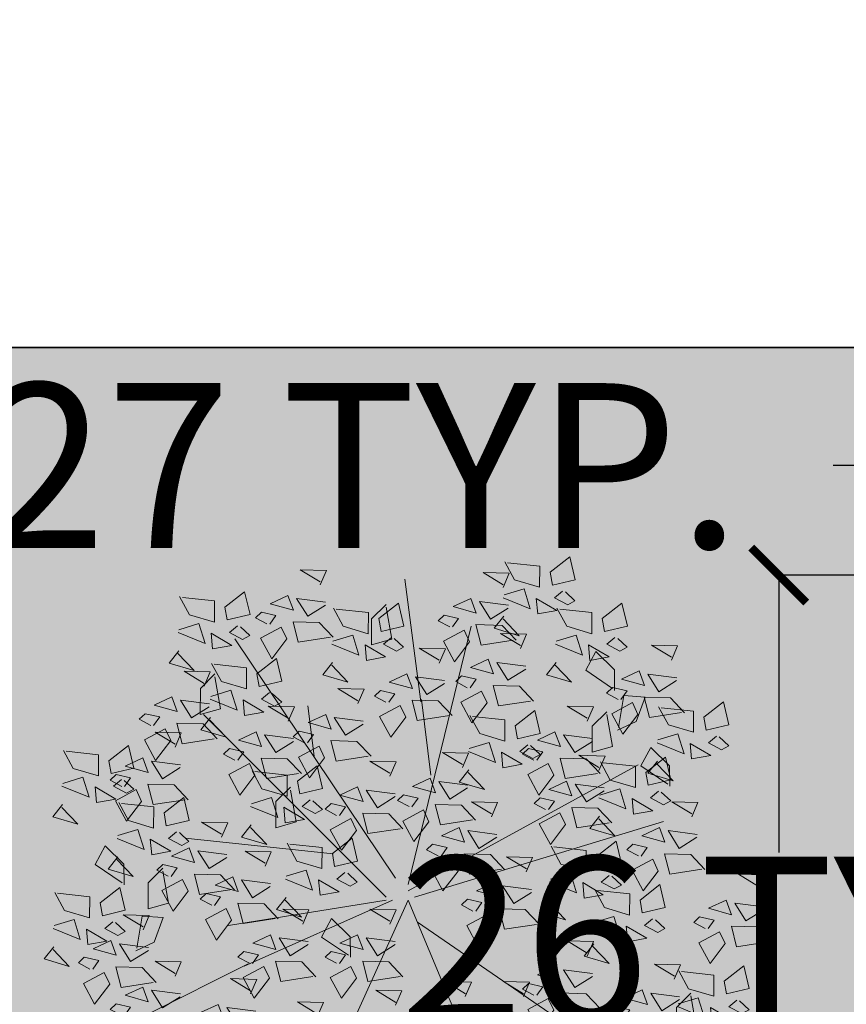
# Model space of a CAD drawing. Units: inches. Extents: x 1704 to 6393, y -157 to 1172.
# Tile 77 of 122: x 1987 to 2017, y 1009 to 1045. Entities that reach past the tile are written whole.
import ezdxf

# ---------------------------------------------------------------- set-up
doc = ezdxf.new("R2010")
doc.units = ezdxf.units.IN
doc.header["$MEASUREMENT"] = 0
for name, color, linetype, lineweight in [('A-ANNO-DIMS', 7, 'Continuous', 13), ('C-PROP', 7, 'Continuous', 35), ('L-shrub', 74, 'Continuous', 18)]:
    doc.layers.add(name, color=color, linetype=linetype, lineweight=lineweight)
doc.layers.add('L-HRDS-PATT', color=9, linetype='Continuous', lineweight=13, true_color=0xc5c1ba)
doc.styles.get("Standard").update_dxf_attribs({"font": 'arial.ttf'})
doc.dimstyles.get("Standard").update_dxf_attribs({"dimtxt": 6, "dimasz": 2, "dimexe": 0.18, "dimexo": 0.0625, "dimgap": 0.09, "dimtad": 0, "dimtih": 1, "dimtoh": 1, "dimdec": 1, "dimzin": 0, "dimdsep": 46, "dimlunit": 3, "dimtxsty": 'Standard', "dimblk": 'ARCHTICK', "dimcen": 0.09, "dimadec": 0, "dimazin": 0, "dimtfac": 1, "dimtdec": 1, "dimtofl": 0, "dimtmove": 0, "dimatfit": 3, "dimfxl": 1, "dimtolj": 1, "dimtzin": 0, "dimarcsym": 0})

# ---------------------------------------------------------------- blocks, each defined once
blk = doc.blocks.new('flower shrub 2')
at = {"layer": 'L-shrub'}
for p, q in [((-106.23, 211.82), (-92.99, 218)), ((-112.6, 194.32), (-106.23, 211.82)), ((-93.69, 216.06), (-97.6, 193.26)), ((-81.12, 192.39), (-66.64, 196.47)), ((-66.64, 196.47), (-66.71, 177.85)), ((71.95, 198.59), (86.43, 202.67)), ((75.99, 175.82), (71.95, 198.59)), ((86.43, 202.67), (86.36, 184.05)), ((-97.6, 193.26), (-112.6, 194.32)), ((-77.07, 169.62), (-81.12, 192.39)), ((86.36, 184.05), (75.99, 173.75)), ((-66.71, 177.85), (-77.08, 167.55)), ((26.45, 165.53), (40.92, 169.61)), ((40.92, 169.61), (40.85, 150.99)), ((-145.24, 163.47), (-130.76, 167.54)), ((-141.2, 140.7), (-145.24, 163.47)), ((-130.76, 167.54), (-130.83, 148.93)), ((-88.72, 152.29), (-88.87, 166.9)), ((-87.4, 165.46), (-68.26, 152.47)), ((30.49, 142.76), (26.45, 165.53)), ((60.21, 144.02), (60.06, 158.64)), ((61.53, 157.19), (80.67, 144.21)), ((-130.83, 148.93), (-141.21, 138.63)), ((-75.44, 139.25), (-88.72, 152.29)), ((-68.26, 152.47), (-75.44, 139.25)), ((40.85, 150.99), (30.48, 140.69)), ((73.5, 130.99), (60.21, 144.02)), ((80.67, 144.21), (73.5, 130.99)), ((-201.09, 93.22), (-186.61, 97.3)), ((-197.05, 70.45), (-201.09, 93.22)), ((-186.61, 97.3), (-186.68, 78.69)), ((-186.68, 78.69), (-197.06, 68.38)), ((45.73, 28.33), (45.58, 42.95)), ((47.06, 41.5), (66.19, 28.51)), ((185.43, 32.08), (198.67, 38.26)), ((197.96, 36.32), (194.06, 13.53)), ((59.02, 15.29), (45.73, 28.33)), ((66.19, 28.51), (59.02, 15.29)), ((179.06, 14.59), (185.43, 32.08)), ((194.06, 13.53), (179.06, 14.59)), ((175.38, 4.39), (189.86, 8.47)), ((189.86, 8.47), (189.78, -10.15)), ((179.42, -18.38), (175.38, 4.39)), ((189.78, -10.15), (179.41, -20.45)), ((207.07, -23.32), (206.92, -8.7)), ((208.4, -10.15), (227.53, -23.13)), ((220.36, -36.35), (207.07, -23.32)), ((227.53, -23.13), (220.36, -36.35)), ((84.36, -53.46), (98.84, -49.38)), ((88.41, -76.23), (84.36, -53.46)), ((98.84, -49.38), (98.77, -68)), ((98.77, -68), (88.4, -78.3)), ((-181.81, -93.56), (-181.96, -78.94)), ((-180.48, -80.39), (-161.34, -93.38)), ((-168.52, -106.6), (-181.81, -93.56)), ((-161.34, -93.38), (-168.52, -106.6)), ((-141.1, -107.17), (-126.62, -103.09)), ((-126.62, -103.09), (-126.7, -121.71)), ((-137.06, -129.94), (-141.1, -107.17)), ((-157.94, -124.93), (-144.7, -118.75)), ((-164.31, -142.42), (-157.94, -124.93)), ((-145.41, -120.69), (-149.31, -143.48)), ((-126.7, -121.71), (-137.07, -132.01)), ((138.15, -134.03), (152.62, -129.95)), ((152.62, -129.95), (152.55, -148.57)), ((142.19, -156.8), (138.15, -134.03)), ((-149.31, -143.48), (-164.31, -142.42)), ((-142.51, -161.74), (-142.65, -147.12)), ((-141.18, -148.57), (-122.04, -161.55)), ((152.55, -148.57), (142.18, -158.87)), ((-129.22, -174.77), (-142.51, -161.74)), ((-122.04, -161.55), (-129.22, -174.77)), ((16.1, -183.61), (30.58, -179.53)), ((30.58, -179.53), (30.51, -198.15)), ((20.14, -206.38), (16.1, -183.61)), ((30.51, -198.15), (20.14, -208.45))]:
    blk.add_line(p, q, dxfattribs=at)
for points in [[(52.15, 237.83), (59.05, 246.56), (41.2, 251.84), (52.74, 239.81)], [(-67.82, 227.5), (-60.92, 236.23), (-78.77, 241.51), (-67.23, 229.48)], [(-39.32, 221.12), (-28.59, 235.29), (-20.71, 220.61), (-35.41, 212.74), (-39.32, 221.12)], [(29.03, 225.28), (27.99, 236.36), (14.33, 233.94), (29.03, 225.28)], [(52.02, 222.79), (37.77, 218.39), (33.35, 232.62), (52.6, 224.77)], [(-90.95, 214.95), (-91.98, 226.03), (-105.64, 223.61), (-90.95, 214.95)], [(10.23, 220.07), (15.95, 224.84), (6.62, 229.76), (1.48, 226.97), (8.24, 220.66)], [(126.62, 210.97), (133.52, 219.7), (115.67, 224.99), (127.2, 212.95)], [(-109.75, 209.74), (-104.02, 214.51), (-113.35, 219.43), (-118.49, 216.64), (-111.73, 210.33)], [(-67.96, 212.46), (-82.2, 208.06), (-86.62, 222.29), (-67.37, 214.44)], [(-70.39, 219.89), (-47.54, 223.41), (-43.79, 208.84), (-62.4, 209.34), (-72.46, 219.95)], [(-27.19, 210.46), (-31.5, 204.37), (-21.21, 202.03), (-16.97, 206.05), (-25.13, 210.4)], [(19.2, 206.65), (5.18, 195.71), (1.34, 211.93), (17.57, 215.74), (19.2, 206.65)], [(49.53, 199.82), (26.54, 202.32), (26.68, 217.36), (44.53, 212.08), (51.52, 199.24)], [(-100.78, 196.32), (-114.8, 185.38), (-118.63, 201.6), (-102.4, 205.41), (-100.78, 196.32)], [(-70.44, 189.49), (-93.43, 191.99), (-93.29, 207.03), (-75.44, 201.75), (-68.45, 188.91)], [(-66.87, 197.06), (-54.24, 204.99), (-46.3, 192.37), (-66.93, 195)], [(16.53, 190.13), (27.26, 204.31), (35.14, 189.63), (20.44, 181.76), (16.53, 190.13)], [(103.49, 198.43), (102.46, 209.5), (88.8, 207.08), (103.49, 198.43)], [(126.48, 195.93), (112.24, 191.53), (107.82, 205.76), (127.07, 197.91)], [(-47.57, 123.92), (-79, 197.93)], [(-44.01, 200.58), (-40.16, 190.14), (-27.58, 196), (-44.01, 200.58)], [(-37.25, 183.93), (-26.52, 198.11), (-18.64, 183.43), (-33.34, 175.56), (-37.25, 183.93)], [(84.69, 193.22), (90.42, 197.99), (81.09, 202.9), (75.95, 200.11), (82.71, 193.8)], [(-136.54, 179.8), (-125.81, 193.98), (-117.93, 179.3), (-132.63, 171.43), (-136.54, 179.8)], [(-14.54, 188.9), (8.31, 192.42), (12.06, 177.85), (-6.55, 178.35), (-16.61, 188.96)], [(124, 172.97), (101.01, 175.46), (101.15, 190.5), (119, 185.22), (125.98, 172.38)], [(-68.32, 182.7), (-45.47, 186.22), (-41.72, 171.65), (-60.33, 172.15), (-70.39, 182.76)], [(-63.13, 182.49), (-67.54, 172.28), (-48.93, 171.78), (-63.18, 180.43)], [(64.56, 171.72), (71.46, 180.45), (53.61, 185.73), (65.15, 173.7)], [(93.66, 179.79), (79.64, 168.86), (75.81, 185.07), (92.04, 188.89), (93.66, 179.79)], [(-167.61, 178.57), (-144.76, 182.09), (-141.01, 167.52), (-159.62, 168.02), (-169.68, 178.63)], [(28.66, 179.47), (24.35, 173.38), (34.64, 171.04), (38.88, 175.06), (30.72, 179.41)], [(66.94, 139.62), (91.63, 182.23)], [(141.1, 161.39), (148, 170.12), (130.14, 175.4), (141.68, 163.37)], [(-124.41, 169.14), (-128.72, 163.05), (-118.43, 160.71), (-114.19, 164.73), (-122.34, 169.08)], [(-78.16, 157.26), (-71.26, 165.99), (-89.12, 171.27), (-77.58, 159.24)], [(-25.12, 173.27), (-29.43, 167.19), (-19.14, 164.84), (-14.9, 168.86), (-23.06, 173.21)], [(-11.02, 166.07), (1.61, 174), (9.54, 161.38), (-11.08, 164.01)], [(11.84, 169.59), (15.69, 159.15), (28.27, 165.01), (11.84, 169.59)], [(41.44, 159.17), (40.4, 170.25), (26.74, 167.83), (41.44, 159.17)], [(-164.09, 155.74), (-151.46, 163.67), (-143.52, 151.05), (-164.15, 153.68)], [(-105.51, 148.81), (-94.78, 162.99), (-86.9, 148.31), (-101.6, 140.44), (-105.51, 148.81)], [(-64.8, 159.87), (-52.17, 167.8), (-44.24, 155.19), (-64.86, 157.81)], [(-41.95, 163.39), (-38.09, 152.95), (-25.52, 158.81), (-41.95, 163.39)], [(22.64, 153.96), (28.36, 158.73), (19.03, 163.65), (13.89, 160.86), (20.65, 154.55)], [(64.43, 156.68), (50.18, 152.28), (45.76, 166.51), (65.01, 158.66)], [(207.29, 148.99), (214.19, 157.72), (196.34, 163.01), (207.88, 150.97)], [(-165.04, 146.93), (-158.14, 155.66), (-175.99, 160.94), (-164.45, 148.91)], [(-141.23, 159.26), (-137.38, 148.82), (-124.8, 154.68), (-141.23, 159.26)], [(-101.29, 144.71), (-102.33, 155.79), (-115.98, 153.37), (-101.29, 144.71)], [(117.97, 148.84), (116.93, 159.92), (103.28, 157.5), (117.97, 148.84)], [(140.96, 146.35), (126.72, 141.95), (122.3, 156.18), (141.55, 148.33)], [(-136.58, 147.58), (-113.73, 151.1), (-109.98, 136.53), (-128.59, 137.03), (-138.65, 147.64)], [(-120.09, 139.5), (-114.36, 144.27), (-123.69, 149.19), (-128.83, 146.4), (-122.07, 140.09)], [(-78.3, 142.22), (-92.54, 137.81), (-96.96, 152.05), (-77.71, 144.2)], [(-7.28, 151.5), (-11.69, 141.29), (6.92, 140.79), (-7.33, 149.44)], [(31.61, 140.54), (17.59, 129.6), (13.76, 145.82), (29.99, 149.63), (31.61, 140.54)], [(61.95, 133.71), (38.95, 136.21), (39.09, 151.25), (56.94, 145.97), (63.93, 133.13)], [(99.17, 143.63), (104.9, 148.4), (95.57, 153.32), (90.43, 150.53), (97.19, 144.22)], [(184.16, 136.45), (183.13, 147.53), (169.47, 145.1), (184.16, 136.45)], [(-188.17, 134.38), (-189.2, 145.46), (-202.86, 143.04), (-188.17, 134.38)], [(-165.18, 131.89), (-179.42, 127.48), (-183.84, 141.72), (-164.59, 133.87)], [(-160.34, 141.17), (-164.76, 130.96), (-146.15, 130.46), (-160.4, 139.11)], [(-61.06, 145.31), (-65.47, 135.09), (-46.86, 134.59), (-61.11, 143.24)], [(138.48, 123.38), (115.49, 125.88), (115.63, 140.92), (133.48, 135.64), (140.46, 122.8)], [(165.36, 131.24), (171.09, 136.01), (161.76, 140.92), (156.62, 138.13), (163.38, 131.82)], [(207.15, 133.95), (192.91, 129.55), (188.49, 143.78), (207.74, 135.93)], [(-206.97, 129.17), (-201.24, 133.94), (-210.57, 138.86), (-215.71, 136.07), (-208.95, 129.76)], [(-111.12, 126.07), (-125.14, 115.14), (-128.97, 131.36), (-112.74, 135.17), (-111.12, 126.07)], [(-80.78, 119.25), (-103.77, 121.75), (-103.63, 136.79), (-85.78, 131.5), (-78.8, 118.66)], [(-93.39, 138.15), (-97.69, 132.06), (-87.4, 129.72), (-83.16, 133.74), (-91.32, 138.09)], [(108.14, 130.21), (94.12, 119.27), (90.29, 135.49), (106.52, 139.3), (108.14, 130.21)], [(93.06, 124.02), (103.79, 138.2), (111.67, 123.52), (96.98, 115.65), (93.06, 124.02)], [(-167.66, 108.92), (-190.65, 111.42), (-190.51, 126.46), (-172.66, 121.17), (-165.67, 108.33)], [(-133.06, 124.75), (-120.43, 132.68), (-112.5, 120.06), (-133.12, 122.69)], [(-110.21, 128.27), (-106.35, 117.83), (-93.78, 123.69), (-110.21, 128.27)], [(37.21, 115.75), (47.94, 129.93), (55.82, 115.25), (41.13, 107.38), (37.21, 115.75)], [(61.99, 122.79), (84.85, 126.31), (88.59, 111.74), (69.98, 112.24), (59.92, 122.85)], [(174.33, 117.81), (160.31, 106.88), (156.48, 123.09), (172.71, 126.91), (174.33, 117.81)], [(204.67, 110.99), (181.68, 113.48), (181.82, 128.52), (199.67, 123.24), (206.65, 110.4)], [(-198, 115.75), (-212.02, 104.81), (-215.85, 121.03), (-199.62, 124.84), (-198, 115.75)], [(-53.8, 109.56), (-43.07, 123.73), (-35.19, 109.05), (-49.89, 101.18), (-53.8, 109.56)], [(-12.43, 109.56), (-1.7, 123.73), (6.18, 109.05), (-8.52, 101.18), (-12.43, 109.56)], [(4.49, 2.24), (58.38, 121.09)], [(140.64, 107.49), (151.37, 121.67), (159.25, 106.99), (144.55, 99.12), (140.64, 107.49)], [(-2.25, 17.94), (-145.94, 116.61)], [(6.14, 114.53), (29, 118.04), (32.74, 103.47), (14.13, 103.98), (4.07, 114.58)], [(105.19, 113.36), (100.89, 107.27), (111.17, 104.93), (115.42, 108.95), (107.26, 113.3)], [(-161.36, 97.16), (-150.63, 111.34), (-142.75, 96.66), (-157.45, 88.79), (-161.36, 97.16)], [(-129.32, 110.18), (-133.73, 99.97), (-115.12, 99.47), (-129.37, 108.12)], [(-84.87, 108.33), (-62.02, 111.85), (-58.27, 97.28), (-76.88, 97.78), (-86.94, 108.38)], [(-43.5, 108.33), (-20.65, 111.85), (-16.9, 97.28), (-35.51, 97.78), (-45.57, 108.38)], [(4.49, 2.24), (-40.41, 109.88)], [(65.51, 99.96), (78.14, 107.89), (86.08, 95.27), (65.46, 97.9)], [(109.57, 106.26), (132.42, 109.78), (136.17, 95.21), (117.56, 95.71), (107.5, 106.32)], [(194.42, 95.09), (205.15, 109.27), (213.03, 94.59), (198.33, 86.72), (194.42, 95.09)], [(-187.79, 91.15), (-180.89, 99.88), (-198.75, 105.16), (-187.21, 93.13)], [(-192.43, 95.93), (-169.58, 99.45), (-165.83, 84.88), (-184.44, 85.38), (-194.5, 95.99)], [(-41.67, 98.9), (-45.98, 92.81), (-35.69, 90.47), (-31.45, 94.49), (-39.6, 98.84)], [(-0.3, 98.9), (-4.61, 92.81), (5.68, 90.47), (9.92, 94.49), (1.76, 98.84)], [(9.66, 91.7), (22.29, 99.62), (30.23, 87.01), (9.61, 89.63)], [(49.34, 105.09), (45.04, 99.01), (55.32, 96.67), (59.57, 100.68), (51.41, 105.04)], [(88.37, 103.48), (92.23, 93.04), (104.8, 98.9), (88.37, 103.48)], [(-99.31, 80.63), (-88.58, 94.81), (-80.7, 80.13), (-95.39, 72.26), (-99.31, 80.63)], [(-81.35, 85.5), (-68.72, 93.43), (-60.78, 80.81), (-81.41, 83.43)], [(-39.98, 85.5), (-27.35, 93.43), (-19.41, 80.81), (-40.04, 83.43)], [(32.52, 95.21), (36.38, 84.78), (48.95, 90.64), (32.52, 95.21)], [(113.09, 83.43), (125.72, 91.36), (133.65, 78.75), (113.03, 81.37)], [(152.77, 96.83), (148.46, 90.75), (158.75, 88.4), (162.99, 92.42), (154.83, 96.77)], [(163.35, 93.87), (186.2, 97.38), (189.95, 82.82), (171.34, 83.32), (161.28, 93.92)], [(-210.92, 78.6), (-211.96, 89.68), (-225.62, 87.26), (-210.92, 78.6)], [(-187.93, 76.11), (-202.17, 71.7), (-206.59, 85.94), (-187.34, 78.09)], [(-149.23, 86.5), (-153.54, 80.42), (-143.25, 78.07), (-139.01, 82.09), (-147.17, 86.44)], [(-58.49, 89.02), (-54.64, 78.58), (-42.06, 84.44), (-58.49, 89.02)], [(-17.12, 89.02), (-13.27, 78.58), (-0.69, 84.44), (-17.12, 89.02)], [(69.26, 85.39), (64.84, 75.18), (83.45, 74.68), (69.2, 83.33)], [(135.94, 86.95), (139.8, 76.51), (152.38, 82.37), (135.94, 86.95)], [(206.55, 84.43), (202.24, 78.35), (212.53, 76.01), (216.77, 80.02), (208.61, 84.38)], [(-229.72, 73.39), (-223.99, 78.16), (-233.32, 83.08), (-238.46, 80.29), (-231.7, 73.98)], [(-188.91, 73.1), (-176.28, 81.03), (-168.35, 68.42), (-188.97, 71.04)], [(-130.38, 79.41), (-107.52, 82.92), (-103.78, 68.35), (-122.39, 68.86), (-132.45, 79.46)], [(118.58, 47.68), (190.43, 83.56)], [(166.87, 71.04), (179.5, 78.96), (187.44, 66.35), (166.81, 68.97)], [(-190.41, 53.14), (-213.4, 55.64), (-213.26, 70.68), (-195.41, 65.39), (-188.43, 52.55)], [(-166.05, 76.62), (-162.2, 66.18), (-149.62, 72.04), (-166.05, 76.62)], [(-77.6, 70.93), (-82.02, 60.72), (-63.41, 60.22), (-77.66, 68.87)], [(-36.23, 70.93), (-40.65, 60.72), (-22.04, 60.22), (-36.29, 68.87)], [(13.41, 77.13), (8.99, 66.92), (27.6, 66.41), (13.35, 75.06)], [(41.35, 57.91), (52.08, 72.09), (59.96, 57.41), (45.26, 49.54), (41.35, 57.91)], [(103.41, 57.91), (114.13, 72.09), (122.01, 57.41), (107.32, 49.54), (103.41, 57.91)], [(189.73, 74.55), (193.58, 64.12), (206.16, 69.98), (189.73, 74.55)], [(217.17, 62.04), (227.9, 76.22), (235.78, 61.54), (221.08, 53.67), (217.17, 62.04)], [(-220.75, 59.96), (-234.77, 49.03), (-238.6, 65.25), (-222.37, 69.06), (-220.75, 59.96)], [(-126.86, 56.58), (-114.23, 64.5), (-106.29, 51.89), (-126.91, 54.51)], [(-87.18, 69.97), (-91.48, 63.89), (-81.2, 61.54), (-76.95, 65.56), (-85.11, 69.92)], [(116.83, 68.87), (112.42, 58.65), (131.03, 58.15), (116.78, 66.8)], [(186.1, 60.81), (208.96, 64.33), (212.7, 49.76), (194.09, 50.26), (184.03, 60.87)], [(-185.17, 58.54), (-189.58, 48.32), (-170.97, 47.82), (-185.22, 56.47)], [(-104, 60.09), (-100.14, 49.66), (-87.57, 55.52), (-104, 60.09)], [(10.28, 56.68), (33.14, 60.2), (36.88, 45.63), (18.27, 46.13), (8.21, 56.74)], [(72.33, 56.68), (95.19, 60.2), (98.94, 45.63), (80.33, 46.13), (70.27, 56.74)], [(170.61, 56.47), (166.2, 46.26), (184.81, 45.75), (170.56, 54.41)], [(15.72, 2.24), (121.24, 49.33)], [(229.3, 51.38), (225, 45.3), (235.28, 42.95), (239.53, 46.97), (231.37, 51.32)], [(256.93, 35.37), (263.83, 44.1), (245.98, 49.38), (257.52, 37.35)], [(-221.35, 33.12), (-210.62, 47.29), (-202.74, 32.61), (-217.44, 24.74), (-221.35, 33.12)], [(-127.81, 33.3), (-120.91, 42.03), (-138.76, 47.31), (-127.22, 35.28)], [(53.48, 47.25), (49.18, 41.16), (59.46, 38.82), (63.71, 42.84), (55.55, 47.19)], [(115.53, 47.25), (111.23, 41.16), (121.51, 38.82), (125.76, 42.84), (117.6, 47.19)], [(189.62, 37.98), (202.25, 45.91), (210.19, 33.29), (189.57, 35.92)], [(-252.42, 31.89), (-229.56, 35.41), (-225.82, 20.84), (-244.43, 21.34), (-254.49, 31.94)], [(-123.11, 42.01), (-127.53, 31.79), (-108.92, 31.29), (-123.17, 39.94)], [(13.8, 33.85), (26.43, 41.78), (34.37, 29.16), (13.74, 31.79)], [(36.66, 37.37), (40.51, 26.93), (53.09, 32.79), (36.66, 37.37)], [(75.86, 33.85), (88.48, 41.78), (96.42, 29.16), (75.8, 31.79)], [(98.71, 37.37), (102.57, 26.93), (115.14, 32.79), (98.71, 37.37)], [(212.48, 41.5), (216.34, 31.06), (228.91, 36.92), (212.48, 41.5)], [(-150.93, 20.75), (-151.97, 31.83), (-165.63, 29.41), (-150.93, 20.75)], [(-127.94, 18.26), (-142.19, 13.86), (-146.61, 28.09), (-127.36, 20.24)], [(-55.87, 20.72), (-45.14, 34.9), (-37.26, 20.22), (-51.96, 12.35), (-55.87, 20.72)], [(130.3, 16.59), (141.02, 30.77), (148.91, 16.09), (134.21, 8.22), (130.3, 16.59)], [(233.81, 22.82), (232.77, 33.9), (219.11, 31.48), (233.81, 22.82)], [(256.8, 20.33), (242.55, 15.92), (238.13, 30.16), (257.38, 22.31)], [(-209.22, 22.46), (-213.52, 16.37), (-203.24, 14.03), (-198.99, 18.05), (-207.15, 22.4)], [(-169.73, 15.55), (-164.01, 20.31), (-173.34, 25.23), (-178.48, 22.44), (-171.72, 16.13)], [(-86.94, 19.49), (-64.08, 23.01), (-60.34, 8.44), (-78.95, 8.94), (-89.01, 19.55)], [(193.37, 23.42), (188.95, 13.2), (207.56, 12.7), (193.31, 21.35)], [(215.01, 17.61), (220.73, 22.38), (211.4, 27.3), (206.26, 24.51), (213.02, 18.2)], [(-248.9, 9.06), (-236.27, 16.99), (-228.33, 4.37), (-248.95, 7)], [(-96.78, 2.31), (-89.88, 11.04), (-107.73, 16.33), (-96.19, 4.29)], [(17.55, 19.28), (13.13, 9.07), (31.74, 8.57), (17.49, 17.22)], [(20.21, 2.24), (132.47, 20.18)], [(79.6, 19.28), (75.19, 9.07), (93.8, 8.57), (79.54, 17.22)], [(91.45, 0.25), (98.35, 8.98), (80.5, 14.26), (92.04, 2.23)], [(99.22, 15.36), (122.08, 18.88), (125.83, 4.31), (107.22, 4.81), (97.16, 15.42)], [(254.32, -2.64), (231.32, -0.14), (231.46, 14.9), (249.31, 9.61), (256.3, -3.23)], [(-226.04, 12.58), (-222.18, 2.14), (-209.61, 8), (-226.04, 12.58)], [(-160.76, 2.12), (-174.78, -8.81), (-178.61, 7.4), (-162.38, 11.22), (-160.76, 2.12)], [(-130.42, -4.7), (-153.42, -2.21), (-153.28, 12.83), (-135.43, 7.55), (-128.44, -5.29)], [(-43.74, 10.06), (-48.04, 3.98), (-37.76, 1.63), (-33.51, 5.65), (-41.67, 10)], [(161.32, -4.07), (172.05, 10.11), (179.93, -4.57), (165.24, -12.44), (161.32, -4.07)], [(223.98, 4.18), (209.96, -6.75), (206.13, 9.47), (222.35, 13.28), (223.98, 4.18)], [(0, 0), (-177.37, -53.82)], [(-119.91, -10.23), (-120.94, 0.84), (-134.6, -1.58), (-119.91, -10.23)], [(-83.42, -3.34), (-70.79, 4.59), (-62.85, -8.02), (-83.47, -5.4)], [(-60.56, 0.18), (-56.71, -10.26), (-44.13, -4.4), (-60.56, 0.18)], [(20.21, 0), (150.43, -130.06)], [(102.75, -7.47), (115.38, 0.46), (123.31, -12.16), (102.69, -9.53)], [(142.42, 5.93), (138.12, -0.16), (148.4, -2.5), (152.65, 1.52), (144.49, 5.87)], [(-245.15, -5.51), (-249.57, -15.72), (-230.96, -16.22), (-245.21, -7.57)], [(-173.77, -18.53), (-163.04, -4.35), (-155.16, -19.03), (-169.86, -26.9), (-173.77, -18.53)], [(4.49, -4.48), (-159.41, -94.18)], [(-138.71, -15.44), (-132.98, -10.67), (-142.31, -5.76), (-147.45, -8.55), (-140.69, -14.86)], [(-96.92, -12.73), (-111.16, -17.13), (-115.58, -2.9), (-96.33, -10.75)], [(-31.05, -18.53), (-20.32, -4.35), (-12.44, -19.03), (-27.13, -26.9), (-31.05, -18.53)], [(68.33, -12.3), (67.29, -1.22), (53.63, -3.64), (68.33, -12.3)], [(91.32, -14.79), (77.07, -19.2), (72.66, -4.96), (91.9, -12.81)], [(125.6, -3.95), (129.46, -14.39), (142.03, -8.53), (125.6, -3.95)], [(130.25, -5.3), (153.11, -1.78), (156.85, -16.35), (138.24, -15.85), (128.18, -5.24)], [(4.49, -8.97), (-40.41, -192.85)], [(13.47, -13.45), (127.98, -183.88)], [(49.53, -17.51), (55.25, -12.74), (45.92, -7.82), (40.78, -10.61), (47.54, -16.92)], [(-204.84, -19.76), (-181.99, -16.24), (-178.24, -30.81), (-196.85, -30.31), (-206.91, -19.7)], [(-129.74, -28.87), (-143.76, -39.8), (-147.59, -23.59), (-131.36, -19.77), (-129.74, -28.87)], [(-99.4, -35.69), (-122.39, -33.2), (-122.25, -18.16), (-104.4, -23.44), (-97.41, -36.28)], [(-79.67, -17.9), (-84.09, -28.12), (-65.48, -28.62), (-79.73, -19.97)], [(-62.12, -19.76), (-39.26, -16.24), (-35.52, -30.81), (-54.13, -30.31), (-64.19, -19.7)], [(88.84, -37.76), (65.84, -35.27), (65.98, -20.22), (83.83, -25.51), (90.82, -38.35)], [(133.77, -28.13), (146.4, -20.2), (154.34, -32.82), (133.72, -30.19)], [(173.45, -14.73), (169.15, -20.81), (179.43, -23.16), (183.68, -19.14), (175.52, -14.79)], [(211.43, -28.68), (218.32, -19.95), (200.47, -14.66), (212.01, -26.7)], [(58.5, -30.94), (44.48, -41.87), (40.65, -25.65), (56.88, -21.84), (58.5, -30.94)], [(106.49, -22.04), (102.08, -32.25), (120.69, -32.75), (106.44, -24.1)], [(156.63, -24.61), (160.49, -35.05), (173.06, -29.19), (156.63, -24.61)], [(-201.32, -42.59), (-188.69, -34.66), (-180.76, -47.28), (-201.38, -44.65)], [(-161.65, -29.19), (-165.95, -35.28), (-155.67, -37.62), (-151.42, -33.6), (-159.58, -29.25)], [(-58.6, -42.59), (-45.97, -34.66), (-38.03, -47.28), (-58.65, -44.65)], [(-18.92, -29.19), (-23.22, -35.28), (-12.94, -37.62), (-8.69, -33.6), (-16.85, -29.25)], [(41.35, -47.45), (52.08, -33.28), (59.96, -47.96), (45.26, -55.83), (41.35, -47.45)], [(57.96, -30.81), (163.48, -42.02)], [(188.3, -41.22), (187.26, -30.14), (173.6, -32.57), (188.3, -41.22)], [(211.29, -43.72), (197.04, -48.12), (192.63, -33.89), (211.88, -41.74)], [(-178.47, -39.07), (-174.61, -49.51), (-162.04, -43.65), (-178.47, -39.07)], [(-107.58, -51.59), (-96.85, -37.41), (-88.97, -52.09), (-103.67, -59.96), (-107.58, -51.59)], [(-35.74, -39.07), (-31.88, -49.51), (-19.31, -43.65), (-35.74, -39.07)], [(-10.36, -53.65), (0.37, -39.48), (8.25, -54.15), (-6.45, -62.02), (-10.36, -53.65)], [(116.28, -51.4), (123.17, -42.67), (105.32, -37.39), (116.86, -49.42)], [(169.5, -46.43), (175.23, -41.66), (165.89, -36.75), (160.76, -39.54), (167.52, -45.85)], [(-131.94, -57.6), (-125.04, -48.87), (-142.9, -43.59), (-131.36, -55.62)], [(10.28, -48.68), (33.14, -45.17), (36.88, -59.73), (18.27, -59.23), (8.21, -48.63)], [(137.52, -42.69), (133.1, -52.91), (151.71, -53.41), (137.46, -44.76)], [(-138.65, -52.81), (-115.8, -49.3), (-112.05, -63.87), (-130.66, -63.36), (-140.72, -52.76)], [(-41.43, -54.88), (-18.58, -51.36), (-14.83, -65.93), (-33.44, -65.43), (-43.5, -54.82)], [(93.15, -63.95), (92.11, -52.87), (78.45, -55.29), (93.15, -63.95)], [(178.47, -59.86), (164.45, -70.79), (160.62, -54.58), (176.85, -50.76), (178.47, -59.86)], [(208.81, -66.68), (185.82, -64.19), (185.95, -49.15), (203.81, -54.43), (210.79, -67.27)], [(194.42, -68.11), (205.15, -53.94), (213.03, -68.62), (198.33, -76.49), (194.42, -68.11)], [(250.73, -65.86), (257.63, -57.13), (239.78, -51.85), (251.31, -63.88)], [(-197.58, -57.16), (-201.99, -67.37), (-183.38, -67.87), (-197.63, -59.22)], [(-155.07, -70.15), (-156.11, -59.07), (-169.77, -61.49), (-155.07, -70.15)], [(-132.08, -72.64), (-146.33, -77.04), (-150.74, -62.81), (-131.49, -70.66)], [(-95.45, -62.25), (-99.76, -68.33), (-89.47, -70.68), (-85.23, -66.66), (-93.39, -62.3)], [(-54.85, -57.16), (-59.27, -67.37), (-40.66, -67.87), (-54.91, -59.22)], [(53.48, -58.12), (49.18, -64.2), (59.46, -66.54), (63.71, -62.52), (55.55, -58.17)], [(74.35, -69.16), (80.08, -64.39), (70.74, -59.47), (65.6, -62.26), (72.37, -68.57)], [(116.14, -66.44), (101.89, -70.85), (97.48, -56.61), (116.73, -64.46)], [(-173.87, -75.36), (-168.14, -70.59), (-177.47, -65.67), (-182.61, -68.46), (-175.85, -74.77)], [(-135.13, -75.64), (-122.5, -67.72), (-114.56, -80.33), (-135.19, -77.71)], [(-37.91, -77.71), (-25.28, -69.78), (-17.35, -82.4), (-37.97, -79.77)], [(1.77, -64.31), (-2.54, -70.4), (7.75, -72.74), (11.99, -68.72), (3.83, -64.37)], [(13.8, -71.51), (26.43, -63.59), (34.37, -76.2), (13.74, -73.58)], [(36.66, -67.99), (40.51, -78.43), (53.09, -72.57), (36.66, -67.99)], [(163.35, -69.34), (186.2, -65.83), (189.95, -80.39), (171.34, -79.89), (161.28, -69.29)], [(227.6, -78.41), (226.56, -67.33), (212.91, -69.75), (227.6, -78.41)], [(-112.27, -72.13), (-108.42, -82.56), (-95.84, -76.7), (-112.27, -72.13)], [(-99.31, -86.71), (-88.58, -72.53), (-80.7, -87.21), (-95.39, -95.08), (-99.31, -86.71)], [(-38.86, -90.66), (-31.96, -81.92), (-49.81, -76.64), (-38.27, -88.67)], [(-15.06, -74.19), (-11.2, -84.63), (1.38, -78.77), (-15.06, -74.19)], [(83.32, -82.58), (69.3, -93.52), (65.47, -77.3), (81.7, -73.49), (83.32, -82.58)], [(113.66, -89.41), (90.67, -86.91), (90.8, -71.87), (108.65, -77.16), (115.64, -90)], [(113.75, -86.71), (124.48, -72.53), (132.36, -87.21), (117.66, -95.08), (113.75, -86.71)], [(208.8, -83.62), (214.53, -78.85), (205.2, -73.93), (200.06, -76.72), (206.82, -83.03)], [(250.59, -80.9), (236.35, -85.31), (231.93, -71.07), (251.18, -78.92)], [(-173.31, -96.85), (-166.41, -88.12), (-184.27, -82.84), (-172.73, -94.87)], [(-164.9, -88.78), (-178.92, -99.72), (-182.75, -83.5), (-166.52, -79.68), (-164.9, -88.78)], [(-134.56, -95.61), (-157.55, -93.11), (-157.42, -78.07), (-139.56, -83.35), (-132.58, -96.19)], [(206.55, -78.77), (202.24, -84.86), (212.53, -87.2), (216.77, -83.18), (208.61, -78.83)], [(-131.39, -90.21), (-135.8, -100.43), (-117.19, -100.93), (-131.44, -92.28)], [(-130.38, -87.94), (-107.52, -84.42), (-103.78, -98.99), (-122.39, -98.48), (-132.45, -87.88)], [(-4.91, -140.69), (-11.65, -86.87)], [(17.55, -86.08), (13.13, -96.29), (31.74, -96.8), (17.49, -88.14)], [(64.1, -99.1), (74.83, -84.93), (82.71, -99.61), (68.02, -107.48), (64.1, -99.1)], [(82.68, -87.94), (105.53, -84.42), (109.28, -98.99), (90.67, -98.48), (80.61, -87.88)], [(166.87, -92.17), (179.5, -84.24), (187.44, -96.86), (166.81, -94.24)], [(189.73, -88.65), (193.58, -99.09), (206.16, -93.23), (189.73, -88.65)], [(217.77, -97.05), (203.75, -107.98), (199.92, -91.76), (216.15, -87.95), (217.77, -97.05)], [(248.11, -103.87), (225.12, -101.38), (225.26, -86.33), (243.11, -91.62), (250.09, -104.46)], [(-87.18, -97.37), (-91.48, -103.45), (-81.2, -105.8), (-76.95, -101.78), (-85.11, -97.42)], [(-61.99, -103.2), (-63.02, -92.12), (-76.68, -94.54), (-61.99, -103.2)], [(-39, -105.7), (-53.24, -110.1), (-57.66, -95.86), (-38.41, -103.72)], [(-34.17, -92.28), (-38.58, -102.49), (-19.97, -102.99), (-34.22, -94.34)], [(33.03, -100.33), (55.89, -96.81), (59.63, -111.38), (41.02, -110.88), (30.96, -100.28)], [(125.88, -97.37), (121.57, -103.45), (131.86, -105.8), (136.1, -101.78), (127.94, -97.42)], [(173.73, -111.5), (184.46, -97.32), (192.34, -112), (177.65, -119.87), (173.73, -111.5)], [(-215.24, -114.61), (-209.51, -109.84), (-218.84, -104.92), (-223.98, -107.71), (-217.22, -114.02)], [(-196.44, -109.4), (-197.48, -98.32), (-211.14, -100.74), (-196.44, -109.4)], [(-173.45, -111.89), (-187.7, -116.3), (-192.11, -102.06), (-172.86, -109.91)], [(-126.86, -110.76), (-114.23, -102.84), (-106.29, -115.45), (-126.91, -112.83)], [(-80.79, -108.41), (-75.06, -103.64), (-84.39, -98.73), (-89.53, -101.51), (-82.77, -107.82)], [(71.43, -100.32), (75.92, -136.2)], [(86.2, -110.76), (98.83, -102.84), (106.76, -115.45), (86.14, -112.83)], [(-104, -107.25), (-100.14, -117.69), (-87.57, -111.82), (-104, -107.25)], [(-41.48, -128.66), (-64.47, -126.17), (-64.33, -111.13), (-46.48, -116.41), (-39.5, -129.25)], [(76.23, -109.76), (71.93, -115.85), (82.21, -118.19), (86.46, -114.17), (78.3, -109.82)], [(109.05, -107.25), (112.91, -117.69), (125.48, -111.82), (109.05, -107.25)], [(142.66, -112.73), (165.52, -109.21), (169.26, -123.78), (150.65, -123.28), (140.59, -112.67)], [(170.61, -106.74), (166.2, -116.95), (184.81, -117.46), (170.56, -108.8)], [(-206.27, -128.04), (-220.29, -138.97), (-224.12, -122.75), (-207.89, -118.94), (-206.27, -128.04)], [(-175.93, -134.86), (-198.92, -132.36), (-198.79, -117.32), (-180.93, -122.61), (-173.95, -135.45)], [(-159.29, -130.09), (-148.56, -115.91), (-140.68, -130.59), (-155.38, -138.46), (-159.29, -130.09)], [(-71.82, -121.84), (-85.84, -132.77), (-89.67, -116.56), (-73.44, -112.74), (-71.82, -121.84)], [(6.19, -128.03), (16.91, -113.85), (24.8, -128.53), (10.1, -136.4), (6.19, -128.03)], [(36.55, -123.16), (49.18, -115.23), (57.12, -127.85), (36.5, -125.22)], [(145.23, -127.84), (152.13, -119.11), (134.28, -113.83), (145.82, -125.86)], [(-123.11, -125.33), (-127.53, -135.55), (-108.92, -136.05), (-123.17, -127.4)], [(-51.73, -138.36), (-41, -124.18), (-33.12, -138.86), (-47.82, -146.73), (-51.73, -138.36)], [(-24.89, -129.25), (-2.03, -125.74), (1.72, -140.31), (-16.89, -139.8), (-26.95, -129.2)], [(59.41, -119.64), (63.27, -130.08), (75.84, -124.22), (59.41, -119.64)], [(89.94, -125.33), (85.53, -135.55), (104.14, -136.05), (89.89, -127.4)], [(185.86, -122.16), (181.56, -128.24), (191.84, -130.59), (196.09, -126.57), (187.93, -122.22)], [(-190.37, -131.32), (-167.51, -127.8), (-163.76, -142.37), (-182.37, -141.87), (-192.43, -131.26)], [(122.11, -140.39), (121.07, -129.31), (107.41, -131.73), (122.11, -140.39)], [(145.1, -142.88), (130.85, -147.29), (126.44, -133.05), (145.68, -140.9)], [(146.18, -135.56), (158.81, -127.63), (166.75, -140.24), (146.13, -137.62)], [(169.04, -132.04), (172.9, -142.48), (185.47, -136.62), (169.04, -132.04)], [(-82.8, -139.58), (-59.95, -136.07), (-56.2, -150.64), (-74.81, -150.13), (-84.87, -139.53)], [(-4.49, -139.03), (6.74, -226.49)], [(18.31, -138.69), (14.01, -144.77), (24.29, -147.12), (28.54, -143.1), (20.38, -138.74)], [(40.3, -137.73), (35.89, -147.94), (54.49, -148.44), (40.24, -139.79)], [(103.31, -145.6), (109.03, -140.83), (99.7, -135.91), (94.56, -138.7), (101.33, -145.01)], [(-186.84, -154.15), (-174.21, -146.22), (-166.28, -158.84), (-186.9, -156.21)], [(-147.17, -140.75), (-151.47, -146.84), (-141.19, -149.18), (-136.94, -145.16), (-145.1, -140.81)], [(-21.36, -152.08), (-8.73, -144.16), (-0.8, -156.77), (-21.42, -154.15)], [(-163.99, -150.63), (-160.13, -161.07), (-147.56, -155.21), (-163.99, -150.63)], [(-100.92, -167.09), (-94.02, -158.36), (-111.87, -153.08), (-100.33, -165.11)], [(-39.6, -149.02), (-43.91, -155.1), (-33.62, -157.44), (-29.38, -153.43), (-37.54, -149.07)], [(1.49, -148.57), (5.35, -159), (17.92, -153.14), (1.49, -148.57)], [(58.36, -167.09), (65.26, -158.36), (47.41, -153.08), (58.94, -165.11)], [(112.28, -159.02), (98.26, -169.96), (94.43, -153.74), (110.66, -149.93), (112.28, -159.02)], [(142.62, -165.85), (119.63, -163.35), (119.76, -148.31), (137.61, -153.6), (144.6, -166.44)], [(149.93, -150.12), (145.52, -160.34), (164.12, -160.84), (149.87, -152.19)], [(-79.28, -162.41), (-66.65, -154.49), (-58.72, -167.1), (-79.34, -164.48)], [(-56.42, -158.9), (-52.57, -169.33), (-39.99, -163.47), (-56.42, -158.9)], [(-39.32, -181.74), (-28.59, -167.56), (-20.71, -182.24), (-35.41, -190.11), (-39.32, -181.74)], [(-17.62, -166.65), (-22.03, -176.87), (-3.42, -177.37), (-17.67, -168.72)], [(167.99, -175.36), (174.89, -166.63), (157.04, -161.34), (168.57, -173.38)], [(-183.1, -168.72), (-187.51, -178.93), (-168.9, -179.43), (-183.15, -170.78)], [(-142.84, -184.85), (-137.12, -180.08), (-146.45, -175.17), (-151.59, -177.95), (-144.83, -184.26)], [(-124.04, -179.64), (-125.08, -168.56), (-138.74, -170.98), (-124.04, -179.64)], [(-101.05, -182.14), (-115.3, -186.54), (-119.71, -172.3), (-100.47, -180.15)], [(16.43, -184.85), (22.16, -180.08), (12.83, -175.17), (7.69, -177.95), (14.45, -184.26)], [(35.23, -179.64), (34.2, -168.56), (20.54, -170.98), (35.23, -179.64)], [(58.22, -182.14), (43.98, -186.54), (39.56, -172.3), (58.81, -180.15)], [(90.99, -183.81), (101.72, -169.63), (109.6, -184.31), (94.91, -192.18), (90.99, -183.81)], [(-75.54, -176.98), (-79.95, -187.19), (-61.34, -187.7), (-75.59, -179.05)], [(-70.39, -182.97), (-47.54, -179.45), (-43.79, -194.02), (-62.4, -193.52), (-72.46, -182.91)], [(59.92, -185.03), (82.78, -181.52), (86.52, -196.09), (67.91, -195.58), (57.85, -184.98)], [(144.86, -187.9), (143.83, -176.83), (130.17, -179.25), (144.86, -187.9)], [(167.85, -190.4), (153.61, -194.8), (149.19, -180.57), (168.44, -188.42)], [(-133.87, -198.28), (-147.89, -209.21), (-151.72, -192.99), (-135.49, -189.18), (-133.87, -198.28)], [(-103.53, -205.1), (-126.52, -202.61), (-126.39, -187.57), (-108.54, -192.85), (-101.55, -205.69)], [(-63.68, -200.15), (-56.78, -191.42), (-74.64, -186.14), (-63.1, -198.17)], [(25.4, -198.28), (11.38, -209.21), (7.55, -192.99), (23.78, -189.18), (25.4, -198.28)], [(55.74, -205.1), (32.75, -202.61), (32.89, -187.57), (50.74, -192.85), (57.72, -205.69)], [(126.06, -193.11), (131.79, -188.35), (122.46, -183.43), (117.32, -186.22), (124.08, -192.53)], [(-27.19, -192.4), (-31.5, -198.49), (-21.21, -200.83), (-16.97, -196.81), (-25.13, -192.46)], [(103.12, -194.47), (98.82, -200.55), (109.1, -202.9), (113.35, -198.88), (105.19, -194.52)], [(165.37, -213.36), (142.38, -210.87), (142.52, -195.83), (160.37, -201.11), (167.35, -213.95)], [(-86.81, -212.7), (-87.85, -201.62), (-101.51, -204.04), (-86.81, -212.7)], [(-66.87, -205.8), (-54.24, -197.87), (-46.3, -210.49), (-66.93, -207.86)], [(-44.01, -202.28), (-40.16, -212.72), (-27.58, -206.86), (-44.01, -202.28)], [(63.44, -207.86), (76.07, -199.94), (84.01, -212.55), (63.39, -209.93)], [(135.03, -206.54), (121.01, -217.47), (117.18, -201.26), (133.41, -197.44), (135.03, -206.54)], [(-105.61, -217.91), (-99.88, -213.14), (-109.21, -208.22), (-114.35, -211.01), (-107.59, -217.32)], [(-63.82, -215.19), (-78.07, -219.59), (-82.48, -205.36), (-63.23, -213.21)], [(86.3, -204.35), (90.16, -214.78), (102.73, -208.92), (86.3, -204.35)], [(-96.64, -231.33), (-110.66, -242.26), (-114.49, -226.05), (-98.26, -222.23), (-96.64, -231.33)], [(-66.3, -238.16), (-89.29, -235.66), (-89.16, -220.62), (-71.3, -225.9), (-64.32, -238.74)], [(-63.13, -220.37), (-67.54, -230.58), (-48.93, -231.08), (-63.18, -222.43)], [(67.19, -222.43), (62.78, -232.65), (81.39, -233.15), (67.13, -224.5)]]:
    blk.add_lwpolyline(points, dxfattribs=at)
blk = doc.blocks.new('_ArchTick')
at = {"color": 0, "linetype": 'ByBlock', "const_width": 0.15}
blk.add_lwpolyline([(-0.5, -0.5), (0.5, 0.5)], dxfattribs=at)
blk = doc.blocks.new('*D80')
at = {"layer": 'A-ANNO-DIMS', "color": 0, "lineweight": -2, "transparency": 16777216}
for p, q in [((2018.966, 1028.916), (2016.966, 1028.916)), ((2018.966, 1025.001), (2018.966, 1029.096)), ((2045.487, 1028.916), (2018.966, 1028.916)), ((2045.487, 1025.001), (2045.487, 1029.096))]:
    blk.add_line(p, q, dxfattribs=at)
at = {"layer": 'Defpoints', "color": 0, "lineweight": -3, "transparency": 16777216}
for p in [(2018.966, 1028.916), (2018.966, 1024.938), (2045.487, 1024.938)]:
    blk.add_point(p, dxfattribs=at)
at = {"layer": 'A-ANNO-DIMS', "color": 0, "lineweight": -2, "transparency": 16777216, "xscale": 2, "yscale": 2, "zscale": 2, "rotation": 180}
blk.add_blockref('_ArchTick', (2018.966, 1028.916), dxfattribs=at)
at = {"layer": 'A-ANNO-DIMS', "color": 0, "lineweight": -2, "transparency": 16777216, "xscale": 2, "yscale": 2, "zscale": 2}
blk.add_blockref('_ArchTick', (2045.487, 1028.916), dxfattribs=at)
at = {"layer": 'A-ANNO-DIMS', "color": 0, "transparency": 16777216, "insert": (1967.173, 1028.916), "char_height": 6, "attachment_point": 5}
blk.add_mtext('\\A1;AUTUMN SHRUB 27 TYP.', dxfattribs=at)
blk = doc.blocks.new('*D81')
at = {"layer": 'A-ANNO-DIMS', "color": 0, "lineweight": -2, "transparency": 16777216}
for p, q in [((2018.903, 1024.938), (2014.807, 1024.938)), ((2014.987, 1024.938), (2014.987, 1014.847)), ((2014.987, 998.449), (2014.987, 1008.54)), ((2018.903, 998.449), (2014.807, 998.449))]:
    blk.add_line(p, q, dxfattribs=at)
at = {"layer": 'Defpoints', "color": 0, "lineweight": -3, "transparency": 16777216}
for p in [(2018.966, 1024.938), (2014.987, 998.449), (2018.966, 998.449)]:
    blk.add_point(p, dxfattribs=at)
at = {"layer": 'A-ANNO-DIMS', "color": 0, "lineweight": -2, "transparency": 16777216, "xscale": 2, "yscale": 2, "zscale": 2}
for p, rotation in [((2014.987, 1024.938), 90), ((2014.987, 998.449), 270)]:
    blk.add_blockref('_ArchTick', p, dxfattribs=dict(at, rotation=rotation))
at = {"layer": 'A-ANNO-DIMS', "color": 0, "transparency": 16777216, "insert": (2014.987, 1011.694), "char_height": 6, "attachment_point": 5}
blk.add_mtext('\\A1;26 TYP.', dxfattribs=at)
blk = doc.blocks.new('*D94')
at = {"layer": 'A-ANNO-DIMS', "color": 0, "lineweight": -2, "transparency": 16777216}
for p, q in [((1898.349, 895.275), (1898.349, 1105.287)), ((1898.349, 1105.107), (1979.39, 1105.107)), ((2073.349, 1105.107), (1992.307, 1105.107)), ((2073.349, 895.275), (2073.349, 1105.287))]:
    blk.add_line(p, q, dxfattribs=at)
at = {"layer": 'Defpoints', "color": 0, "lineweight": -3, "transparency": 16777216}
for p in [(2073.349, 1105.107), (1898.349, 895.213), (2073.349, 895.213)]:
    blk.add_point(p, dxfattribs=at)
at = {"layer": 'A-ANNO-DIMS', "color": 0, "lineweight": -2, "transparency": 16777216, "xscale": 2, "yscale": 2, "zscale": 2, "rotation": 180}
blk.add_blockref('_ArchTick', (1898.349, 1105.107), dxfattribs=at)
at = {"layer": 'A-ANNO-DIMS', "color": 0, "lineweight": -2, "transparency": 16777216, "xscale": 2, "yscale": 2, "zscale": 2}
blk.add_blockref('_ArchTick', (2073.349, 1105.107), dxfattribs=at)
at = {"layer": 'A-ANNO-DIMS', "color": 0, "transparency": 16777216, "insert": (1985.849, 1105.107), "char_height": 6, "attachment_point": 5}
blk.add_mtext('\\A1;175', dxfattribs=at)

msp = doc.modelspace()

# ---------------------------------------------------------------- hatches: boundary and pattern name
at = {"layer": 'L-HRDS-PATT', "transparency": 33554643}
h = msp.add_hatch(color=256, dxfattribs=at)
h.dxf.hatch_style = 1
h.paths.add_polyline_path([(2065.589, 1033.213), (1898.349, 1033.213), (1898.349, 895.213), (2065.589, 895.213)])

# ---------------------------------------------------------------- linework, layer by layer
at = {"layer": 'C-PROP'}
msp.add_line((2723.349, 1033.213), (1898.349, 1033.213), dxfattribs=at)

# ---------------------------------------------------------------- block references
at = {"layer": 'L-shrub', "xscale": 0.0510581485411622, "yscale": 0.0510581485411622, "zscale": 0.0510581485411622, "rotation": 180}
msp.add_blockref('flower shrub 2', (2001.734, 1013.227), dxfattribs=at)

# ---------------------------------------------------------------- dimensions: what is measured, and where the dimension line sits
at = {"layer": 'A-ANNO-DIMS'}
dim = msp.add_linear_dim(base=(2073.349, 1105.107), p1=(1898.349, 895.213), p2=(2073.349, 895.213), dimstyle='Standard', override={"dimdec": 0, "dimlfac": 1, "dimrnd": 0, "dimzin": 0, "dimdsep": 46, "dimlunit": 2}, dxfattribs=at)
dim.commit()
dim.dimension.update_dxf_attribs({"geometry": '*D94', "text_midpoint": (1985.849, 1105.107)})
for base, p1, p2, angle, text, picture, middle in [((2018.966, 1028.916), (2045.487, 1024.938), (2018.966, 1024.938), 180, 'AUTUMN SHRUB <> TYP.', '*D80', (1967.173, 1028.916)), ((2014.987, 998.449), (2018.966, 1024.938), (2018.966, 998.449), 270, '<> TYP.', '*D81', (2014.987, 1011.694))]:
    dim = msp.add_linear_dim(base=base, p1=p1, p2=p2, angle=angle, text=text, dimstyle='Standard', override={"dimdec": 0, "dimlfac": 1, "dimrnd": 0, "dimzin": 0, "dimdsep": 46, "dimlunit": 2}, dxfattribs=at)
    dim.commit()
    dim.dimension.update_dxf_attribs({"geometry": picture, "text_midpoint": middle})

doc.saveas('drawing.dxf')
